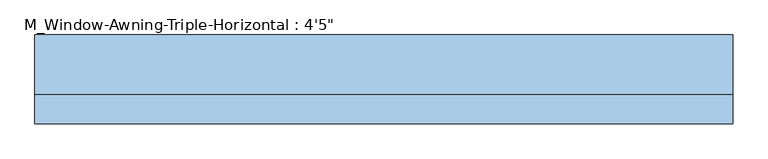
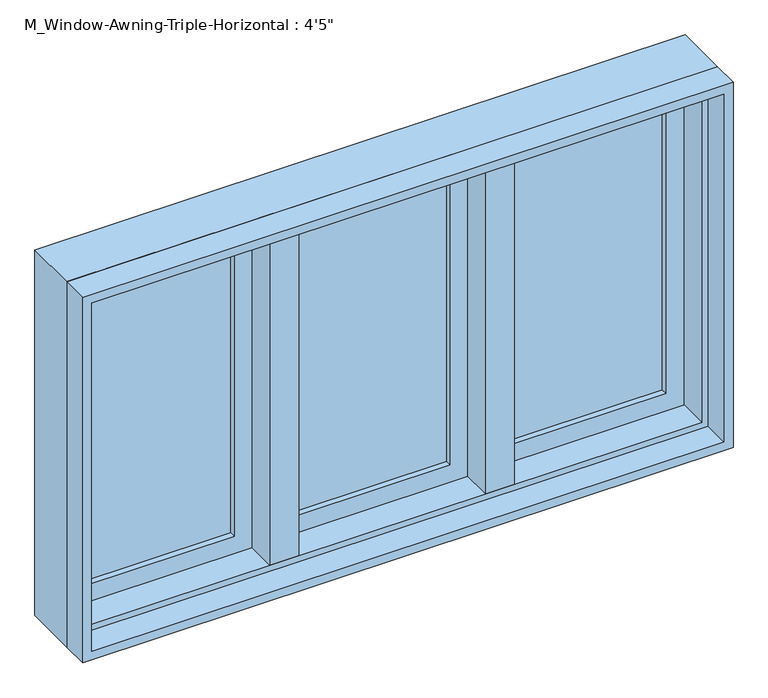
"""IFC4 building model written with IfcOpenShell, lengths in millimetres: window geometry."""

from ifc_helpers import new_model, si_unit, frame, origin, place, context, project, spatial, polyline, outline, extrude, faceted_brep, source, transform, mapped, element, save


def window_61697a4f(model_context):
    return source(origin(), model_context, "Body", "SolidModel", [
        faceted_brep([(641.35, 44.45, 1668.25), (641.35, -19.05, 1668.25), (-641.35, -19.05, 1668.25), (-641.35, 44.45, 1668.25), (660.4, 95.25, 1687.3), (660.4, 44.45, 1687.3), (-660.4, 44.45, 1687.3), (-660.4, 95.25, 1687.3), (673.1, -19.05, 1700.0), (673.1, 95.25, 1700.0), (-673.1, 95.25, 1700.0), (-673.1, -19.05, 1700.0), (-641.35, -19.05, 931.75), (-641.35, 44.45, 931.75), (-660.4, 44.45, 912.7), (-660.4, 95.25, 912.7), (-673.1, 95.25, 900.0), (-673.1, -19.05, 900.0), (641.35, -19.05, 931.75), (641.35, 44.45, 931.75), (660.4, 44.45, 912.7), (660.4, 95.25, 912.7), (673.1, 95.25, 900.0), (673.1, -19.05, 900.0)], [[[0, 1, 2, 3]], [[4, 5, 6, 7]], [[8, 9, 10, 11]], [[3, 2, 12, 13]], [[7, 6, 14, 15]], [[11, 10, 16, 17]], [[13, 12, 18, 19]], [[15, 14, 20, 21]], [[17, 16, 22, 23]], [[11, 17, 23, 8], [1, 18, 12, 2]], [[19, 18, 1, 0]], [[5, 20, 14, 6], [3, 13, 19, 0]], [[21, 20, 5, 4]], [[23, 22, 9, 8]], [[9, 22, 16, 10], [7, 15, 21, 4]]]),
        extrude(outline(polyline([(1700.0, -673.1), (900.0, -673.1), (900.0, 673.1), (1700.0, 673.1), (1700.0, -673.1)]), holes=[polyline([(1680.95, 654.05), (919.05, 654.05), (919.05, -654.05), (1680.95, -654.05), (1680.95, 654.05)])]), frame((0.0, -76.2, 0.0), z_axis=(0.0, 1.0, 0.0), x_axis=(0.0, 0.0, 1.0)), (0.0, 0.0, 1.0), 57.15),
        extrude(outline(polyline([(912.7, 660.4), (1687.3, 660.4), (1687.3, 232.8333333), (912.7, 232.8333333), (912.7, 660.4)]), holes=[polyline([(969.85, 289.9833333), (1630.15, 289.9833333), (1630.15, 603.25), (969.85, 603.25), (969.85, 289.9833333)])]), frame((0.0, 44.45, 0.0), z_axis=(0.0, 1.0, 0.0), x_axis=(0.0, 0.0, 1.0)), (0.0, 0.0, 1.0), 44.45),
        extrude(outline(polyline([(1687.3, -660.4), (912.7, -660.4), (912.7, -232.8333333), (1687.3, -232.8333333), (1687.3, -660.4)]), holes=[polyline([(1630.15, -289.9833333), (969.85, -289.9833333), (969.85, -603.25), (1630.15, -603.25), (1630.15, -289.9833333)])]), frame((0.0, 44.45, 0.0), z_axis=(0.0, 1.0, 0.0), x_axis=(0.0, 0.0, 1.0)), (0.0, 0.0, 1.0), 44.45),
        extrude(outline(polyline([(603.25, 76.2), (603.25, 69.85), (289.9833333, 69.85), (289.9833333, 76.2), (603.25, 76.2)])), frame((0.0, 0.0, 969.85), z_axis=(0.0, 0.0, 1.0), x_axis=(1.0, 0.0, 0.0)), (0.0, 0.0, 1.0), 660.3),
        extrude(outline(polyline([(289.9833333, 57.15), (289.9833333, 63.5), (603.25, 63.5), (603.25, 57.15), (289.9833333, 57.15)])), frame((0.0, 0.0, 969.85), z_axis=(0.0, 0.0, 1.0), x_axis=(1.0, 0.0, 0.0)), (0.0, 0.0, 1.0), 660.3),
        extrude(outline(polyline([(-289.9833333, 76.2), (-289.9833333, 69.85), (-603.25, 69.85), (-603.25, 76.2), (-289.9833333, 76.2)])), frame((0.0, 0.0, 969.85), z_axis=(0.0, 0.0, 1.0), x_axis=(1.0, 0.0, 0.0)), (0.0, 0.0, 1.0), 660.3),
        extrude(outline(polyline([(-603.25, 57.15), (-603.25, 63.5), (-289.9833333, 63.5), (-289.9833333, 57.15), (-603.25, 57.15)])), frame((0.0, 0.0, 969.85), z_axis=(0.0, 0.0, 1.0), x_axis=(1.0, 0.0, 0.0)), (0.0, 0.0, 1.0), 660.3),
        extrude(outline(polyline([(156.6333333, 76.2), (156.6333333, 69.85), (-156.6333333, 69.85), (-156.6333333, 76.2), (156.6333333, 76.2)])), frame((0.0, 0.0, 969.85), z_axis=(0.0, 0.0, 1.0), x_axis=(1.0, 0.0, 0.0)), (0.0, 0.0, 1.0), 660.3),
        extrude(outline(polyline([(-156.6333333, 57.15), (-156.6333333, 63.5), (156.6333333, 63.5), (156.6333333, 57.15), (-156.6333333, 57.15)])), frame((0.0, 0.0, 969.85), z_axis=(0.0, 0.0, 1.0), x_axis=(1.0, 0.0, 0.0)), (0.0, 0.0, 1.0), 660.3),
        extrude(outline(polyline([(912.7, 213.7833333), (1687.3, 213.7833333), (1687.3, -213.7833333), (912.7, -213.7833333), (912.7, 213.7833333)]), holes=[polyline([(969.85, -156.6333333), (1630.15, -156.6333333), (1630.15, 156.6333333), (969.85, 156.6333333), (969.85, -156.6333333)])]), frame((0.0, 44.45, 0.0), z_axis=(0.0, 1.0, 0.0), x_axis=(0.0, 0.0, 1.0)), (0.0, 0.0, 1.0), 44.45),
        faceted_brep([(213.7833333, 44.45, 1687.3), (193.2731995, 44.45, 1687.3), (193.2731995, -19.05, 1687.3), (253.3434672, -19.05, 1687.3), (253.3434672, 44.45, 1687.3), (232.8333333, 44.45, 1687.3), (232.8333333, 95.25, 1687.3), (213.7833333, 95.25, 1687.3), (213.7833333, 95.25, 912.7), (232.8333333, 95.25, 912.7), (232.8333333, 66.675, 912.7), (213.7833333, 66.675, 912.7), (213.7833333, 44.45, 1680.95), (193.2731995, 44.45, 1680.95), (213.7833333, 44.45, 1668.25), (213.7833333, 44.45, 931.75), (193.2731995, 44.45, 931.75), (193.2731995, 44.45, 1668.25), (193.2731995, -19.05, 1680.95), (193.2731995, -19.05, 931.75), (193.2731995, -19.05, 1668.25), (253.3434672, -19.05, 1680.95), (253.3434672, -19.05, 931.75), (253.3434672, -19.05, 1668.25), (253.3434672, 44.45, 1680.95), (253.3434672, 44.45, 931.75), (253.3434672, 44.45, 1668.25), (232.8333333, 44.45, 1680.95), (232.8333333, 44.45, 931.75), (232.8333333, 44.45, 1668.25), (232.8333333, 66.675, 1680.95), (232.8333333, 66.675, 1668.25), (232.8333333, 66.675, 931.75), (213.7833333, 66.675, 931.75), (213.7833333, 66.675, 1668.25), (213.7833333, 66.675, 1680.95)], [[[0, 1, 2, 3, 4, 5, 6, 7]], [[8, 9, 10, 11]], [[1, 0, 12, 13]], [[14, 15, 16, 17]], [[2, 1, 13, 18]], [[17, 16, 19, 20]], [[3, 2, 18, 21]], [[20, 19, 22, 23]], [[4, 3, 21, 24]], [[23, 22, 25, 26]], [[5, 4, 24, 27]], [[26, 25, 28, 29]], [[6, 5, 27, 30, 31, 29, 28, 32, 10, 9]], [[0, 7, 8, 11, 33, 15, 14, 34, 35, 12]], [[30, 35, 34, 31]], [[32, 33, 11, 10]], [[35, 30, 27, 24, 21, 18, 13, 12]], [[31, 34, 14, 17, 20, 23, 26, 29]], [[33, 32, 28, 25, 22, 19, 16, 15]], [[7, 6, 9, 8]]]),
        faceted_brep([(-232.8333333, 44.45, 1687.3), (-253.3434672, 44.45, 1687.3), (-253.3434672, -19.05, 1687.3), (-193.2731995, -19.05, 1687.3), (-193.2731995, 44.45, 1687.3), (-213.7833333, 44.45, 1687.3), (-213.7833333, 95.25, 1687.3), (-232.8333333, 95.25, 1687.3), (-232.8333333, 95.25, 912.7), (-213.7833333, 95.25, 912.7), (-213.7833333, 66.675, 912.7), (-232.8333333, 66.675, 912.7), (-253.3434672, 44.45, 1680.95), (-253.3434672, -19.05, 1680.95), (-253.3434672, 44.45, 1668.25), (-253.3434672, 44.45, 931.75), (-253.3434672, -19.05, 931.75), (-253.3434672, -19.05, 1668.25), (-193.2731995, -19.05, 1680.95), (-193.2731995, -19.05, 931.75), (-193.2731995, -19.05, 1668.25), (-193.2731995, 44.45, 1680.95), (-193.2731995, 44.45, 931.75), (-193.2731995, 44.45, 1668.25), (-213.7833333, 44.45, 1680.95), (-213.7833333, 66.675, 1680.95), (-213.7833333, 66.675, 1668.25), (-213.7833333, 44.45, 1668.25), (-213.7833333, 44.45, 931.75), (-213.7833333, 66.675, 931.75), (-232.8333333, 66.675, 931.75), (-232.8333333, 44.45, 931.75), (-232.8333333, 44.45, 1668.25), (-232.8333333, 66.675, 1668.25), (-232.8333333, 66.675, 1680.95), (-232.8333333, 44.45, 1680.95)], [[[0, 1, 2, 3, 4, 5, 6, 7]], [[8, 9, 10, 11]], [[2, 1, 12, 13]], [[14, 15, 16, 17]], [[3, 2, 13, 18]], [[17, 16, 19, 20]], [[4, 3, 18, 21]], [[20, 19, 22, 23]], [[6, 5, 24, 25, 26, 27, 28, 29, 10, 9]], [[0, 7, 8, 11, 30, 31, 32, 33, 34, 35]], [[25, 34, 33, 26]], [[29, 30, 11, 10]], [[34, 25, 24, 21, 18, 13, 12, 35]], [[26, 33, 32, 14, 17, 20, 23, 27]], [[30, 29, 28, 22, 19, 16, 15, 31]], [[1, 0, 35, 12]], [[15, 14, 32, 31]], [[5, 4, 21, 24]], [[28, 27, 23, 22]], [[7, 6, 9, 8]]]),
    ])


if __name__ == "__main__":
    model = new_model("IFC4")
    model_context = context("Model", 3, world=origin())
    ifc_project = project(units=[si_unit("LENGTHUNIT", "METRE", prefix="MILLI")], contexts=[model_context])
    site = spatial("IfcSite", under=ifc_project)
    building = spatial("IfcBuilding", under=site)
    placement = place(None, origin())
    window_shape = window_61697a4f(model_context)
    element("IfcWindow", 1, ObjectType="M_Window-Awning-Triple-Horizontal : 4'5\"", at=placement, inside=building, context=model_context, shape_type="MappedRepresentation", body=[
        mapped(window_shape, transform((0.0, 0.0, 0.0), x_axis=(1.0, 0.0, 0.0), y_axis=(0.0, 1.0, 0.0), z_axis=(0.0, 0.0, 1.0))),
    ])
    save(model, "model.ifc")

# Revit data of these elements
# Type "M_Window-Awning-Triple-Horizontal : 4'5\""
#   Type Mark = "15"
#   Fire Rating = "0.5h"
#   Assembly Code = "B2020100"
#   Analytic Construction = "Double glazing - domestic"
#   Window Inset [instance default] = 0' - 0"
#   Wall Thickness [instance default] = 0' - 5.90551"
#   Muntin Width = 1' - 0.33333"
#   Visual Light Transmittance = 0.81
#   Thermal Resistance (R) = 1.8146 (h·ft²·°F)/BTU
#   Solar Heat Gain Coefficient = 0.76
#   One Third Width = 1' - 5.66667"
#   Sash Width = 1' - 4.83333"
#   Rough Width = 4' - 5.59055"
#   Rough Height = 2' - 8.08661"
#   Interior Wall Closure [instance default] = 0' - 2.15551"
#   Height = 2' - 7.49606"
#   Heat Transfer Coefficient (U) = 0.5511 BTU/(h·ft²·°F)
#   Muntin Height = 2' - 1.99606"
#   Frame Extension [instance default] = 0' - 0 1/4"
#   Exterior Wall Closure [instance default] = 0' - 1 1/4"
#   Extension Jamb [instance default] = 0' - 2.15551"
#   Default Sill Height = 2' - 11.43307"
#   Width = 4' - 5"
#   Middle Muntin Visibility = yes
#   Side Muntin Visibility = yes
#   Interior Trim Visibility [instance default] = yes
#   Exterior Trim Visibility [instance default] = yes
#   Extension Jamb Visibility [instance default] = yes
#   Muntin Pattern = M_Muntin Pattern_2x2 : M_Muntin Pattern_2x2
#   Interior Trim Material = Wood - Stained
#   Interior Trim = M_Trim-Window-Interior-Flat : Picture Frame
#   Interior Frame Material = Wood - Stained
#   Glass Panel Material = Glass
#   Exterior Trim Material = Clad - White
#   Exterior Trim = M_Trim-Window-Exterior-Flat : with Sill
#   Exterior Frame Material = Clad - White
#   Wall Closure = (empty or 0)
# Element 1 (IfcWindow, "M_Window-Awning-Triple-Horizontal : 4'5\"")
#   Wall Thickness = 0' - 6"
#   Extension Jamb = 0' - 2 1/4"
#   Materials on its faces: "Wood - Stained", "Glass", "Clad - White"
# Materials
#   "Wood - Stained": class "Wood", colour RGB 227 170 128, transparency 0, Cost = 0
#   "Glass": class "Glass", colour RGB 218 227 224, transparency 0.85, Description = "Soda Lime Glass", Cost = 0
#   "Clad - White": class "Wood", colour RGB 242 242 238, transparency 0, Cost = 0
